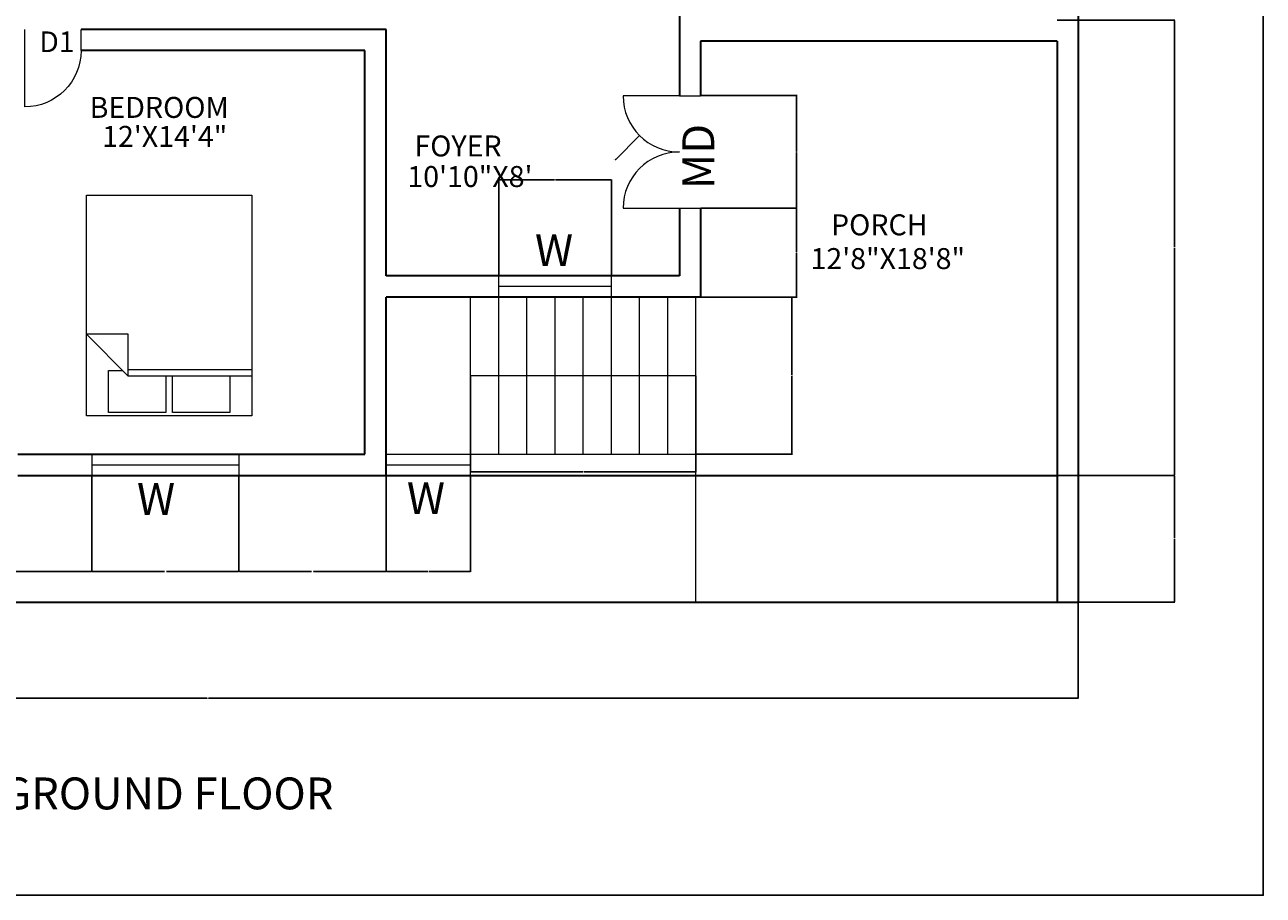
# Model space of a CAD drawing. Units: feet. Extents: x 1755 to 2628, y 1710 to 2329.
# Tile 2 of 4: x 2100 to 2628, y 1710 to 2081. Entities that reach past the tile are written whole.
import ezdxf

# ---------------------------------------------------------------- set-up
doc = ezdxf.new("R2010")
doc.units = ezdxf.units.FT
for name, color, linetype, lineweight in [('A-ANNO-DIMS', 2, 'Continuous', 18), ('A-ANNO-TEXT', 7, 'Continuous', 18), ('A-ANNO-TTLB', 7, 'Continuous', 25), ('A-AREA-IDEN', 7, 'Continuous', 18), ('A-DOOR', 3, 'Continuous', 18), ('A-FLOR-STRS', 7, 'Continuous', 18), ('A-FURN', 8, 'Continuous', 18), ('A-GLAZ', 4, 'Continuous', 18), ('A-WALL', 7, 'Continuous', 35)]:
    doc.layers.add(name, color=color, linetype=linetype, lineweight=lineweight)
doc.styles.get("Standard").update_dxf_attribs({"font": 'arial.ttf'})
doc.dimstyles.get("Standard").update_dxf_attribs({"dimtxt": 0.18, "dimasz": 0.18, "dimexe": 0.18, "dimexo": 0.0625, "dimgap": 0.09, "dimtad": 0, "dimtih": 1, "dimtoh": 1, "dimdec": 4, "dimzin": 0, "dimdsep": 46, "dimtxsty": 'Standard', "dimcen": 0.09, "dimadec": 0, "dimazin": 0, "dimtfac": 1, "dimtdec": 4, "dimtofl": 0, "dimtmove": 0, "dimatfit": 3, "dimfxl": 1, "dimtolj": 1, "dimtzin": 0, "dimarcsym": 0})

# ---------------------------------------------------------------- blocks, each defined once
blk = doc.blocks.new('Bed - Queen')
for p, q in [((0, -80.00003), (0, 0)), ((0, 0), (59.99999, 0)), ((59.99999, 0), (59.99999, -80.00003)), ((7.99999, -1.2), (28.79998, -1.2)), ((7.99999, -14.4), (7.99999, -1.2)), ((28.79998, -1.2), (28.79998, -14.4)), ((31.19999, -1.2), (51.99999, -1.2)), ((31.19999, -14.4), (31.19999, -1.2)), ((51.99999, -1.2), (51.99999, -16.4)), ((0, -14.4), (44.8, -14.4)), ((44.8, -16.8), (0, -16.8)), ((59.99999, -29.6), (44.8, -14.4)), ((44.8, -14.4), (44.8, -29.6)), ((51.99999, -16.4), (46.79936, -16.4)), ((44.8, -29.6), (59.99999, -29.6)), ((59.99999, -80.00003), (0, -80.00003))]:
    blk.add_line(p, q)
blk = doc.blocks.new('DOOR-SINGLE-SWING')
for p, q in [((0, 33), (0, 0)), ((24, 9), (24, 0))]:
    blk.add_line(p, q)
blk.add_arc((0, 9), 24, 0, 90)
blk = doc.blocks.new('*D22')
at = {"layer": 'A-ANNO-DIMS', "color": 0, "lineweight": -2, "transparency": 16777216}
for p, q in [((1806.89, 1834.75), (1806.89, 1793.69)), ((2548.89, 1834.75), (2548.89, 1793.69)), ((1807.07, 1793.87), (2177.6, 1793.87)), ((2548.71, 1793.87), (2178.18, 1793.87))]:
    blk.add_line(p, q, dxfattribs=at)
at = {"layer": 'A-ANNO-DIMS', "color": 0, "transparency": 16777216}
for points in [[(1807.07, 1793.9), (1807.07, 1793.84), (1806.89, 1793.87)], [(2548.71, 1793.9), (2548.71, 1793.84), (2548.89, 1793.87)]]:
    blk.add_solid(points, dxfattribs=at)
at = {"layer": 'Defpoints', "color": 0, "transparency": 16777216}
for p in [(1806.89, 1834.82), (2548.89, 1834.82), (2548.89, 1793.87)]:
    blk.add_point(p, dxfattribs=at)
at = {"layer": 'A-ANNO-DIMS', "color": 0, "transparency": 16777216, "insert": (2177.89, 1793.87), "char_height": 0.18, "attachment_point": 5}
blk.add_mtext('\\A1;742', dxfattribs=at)
blk = doc.blocks.new('*D34')
at = {"layer": 'A-ANNO-DIMS', "color": 0, "lineweight": -2, "transparency": 16777216}
for p, q in [((2539.95, 2082.82), (2590.02, 2082.82)), ((2589.84, 2082.64), (2589.84, 1986)), ((2589.84, 1889), (2589.84, 1985.63)), ((2539.95, 1888.82), (2590.02, 1888.82))]:
    blk.add_line(p, q, dxfattribs=at)
at = {"layer": 'A-ANNO-DIMS', "color": 0, "transparency": 16777216}
for points in [[(2589.81, 2082.64), (2589.87, 2082.64), (2589.84, 2082.82)], [(2589.81, 1889), (2589.87, 1889), (2589.84, 1888.82)]]:
    blk.add_solid(points, dxfattribs=at)
at = {"layer": 'Defpoints', "color": 0, "transparency": 16777216}
for p in [(2539.89, 2082.82), (2539.89, 1888.82), (2589.84, 1888.82)]:
    blk.add_point(p, dxfattribs=at)
at = {"layer": 'A-ANNO-DIMS', "color": 0, "transparency": 16777216, "insert": (2589.84, 1985.82), "char_height": 0.18, "attachment_point": 5}
blk.add_mtext('\\A1;194', dxfattribs=at)
blk = doc.blocks.new('*D35')
at = {"layer": 'A-ANNO-DIMS', "color": 0, "lineweight": -2, "transparency": 16777216}
for p, q in [((2539.95, 1888.82), (2590.02, 1888.82)), ((2589.84, 1888.64), (2589.84, 1862)), ((2589.84, 1835), (2589.84, 1861.63)), ((2539.95, 1834.82), (2590.02, 1834.82))]:
    blk.add_line(p, q, dxfattribs=at)
at = {"layer": 'A-ANNO-DIMS', "color": 0, "transparency": 16777216}
for points in [[(2589.81, 1888.64), (2589.87, 1888.64), (2589.84, 1888.82)], [(2589.81, 1835), (2589.87, 1835), (2589.84, 1834.82)]]:
    blk.add_solid(points, dxfattribs=at)
at = {"layer": 'Defpoints', "color": 0, "transparency": 16777216}
for p in [(2539.89, 1888.82), (2539.89, 1834.82), (2589.84, 1834.82)]:
    blk.add_point(p, dxfattribs=at)
at = {"layer": 'A-ANNO-DIMS', "color": 0, "transparency": 16777216, "insert": (2589.84, 1861.82), "char_height": 0.18, "attachment_point": 5}
blk.add_mtext('\\A1;54', dxfattribs=at)
blk = doc.blocks.new('*D40')
at = {"layer": 'A-ANNO-DIMS', "color": 0, "lineweight": -2, "transparency": 16777216}
for p, q in [((2035.77, 1888.75), (2035.77, 1847.69)), ((2128.5, 1888.75), (2128.5, 1847.69)), ((2035.95, 1847.87), (2081.75, 1847.87)), ((2128.32, 1847.87), (2082.53, 1847.87))]:
    blk.add_line(p, q, dxfattribs=at)
at = {"layer": 'A-ANNO-DIMS', "color": 0, "transparency": 16777216}
for points in [[(2035.95, 1847.9), (2035.95, 1847.84), (2035.77, 1847.87)], [(2128.32, 1847.9), (2128.32, 1847.84), (2128.5, 1847.87)]]:
    blk.add_solid(points, dxfattribs=at)
at = {"layer": 'Defpoints', "color": 0, "transparency": 16777216}
for p in [(2035.77, 1888.82), (2128.5, 1888.82), (2035.77, 1847.87)]:
    blk.add_point(p, dxfattribs=at)
at = {"layer": 'A-ANNO-DIMS', "color": 0, "transparency": 16777216, "insert": (2082.14, 1847.87), "char_height": 0.18, "attachment_point": 5}
blk.add_mtext('\\A1;92.73', dxfattribs=at)
blk = doc.blocks.new('*D41')
at = {"layer": 'A-ANNO-DIMS', "color": 0, "lineweight": -2, "transparency": 16777216}
for p, q in [((2128.5, 1888.75), (2128.5, 1847.69)), ((2191.17, 1888.75), (2191.17, 1847.69)), ((2128.68, 1847.87), (2159.44, 1847.87)), ((2190.99, 1847.87), (2160.23, 1847.87))]:
    blk.add_line(p, q, dxfattribs=at)
at = {"layer": 'A-ANNO-DIMS', "color": 0, "transparency": 16777216}
for points in [[(2128.68, 1847.9), (2128.68, 1847.84), (2128.5, 1847.87)], [(2190.99, 1847.9), (2190.99, 1847.84), (2191.17, 1847.87)]]:
    blk.add_solid(points, dxfattribs=at)
at = {"layer": 'Defpoints', "color": 0, "transparency": 16777216}
for p in [(2128.5, 1888.82), (2191.17, 1888.82), (2128.5, 1847.87)]:
    blk.add_point(p, dxfattribs=at)
at = {"layer": 'A-ANNO-DIMS', "color": 0, "transparency": 16777216, "insert": (2159.83, 1847.87), "char_height": 0.18, "attachment_point": 5}
blk.add_mtext('\\A1;62.66', dxfattribs=at)
blk = doc.blocks.new('*D42')
at = {"layer": 'A-ANNO-DIMS', "color": 0, "lineweight": -2, "transparency": 16777216}
for p, q in [((2191.17, 1888.75), (2191.17, 1847.69)), ((2253.89, 1888.75), (2253.89, 1847.69)), ((2191.35, 1847.87), (2222.13, 1847.87)), ((2253.71, 1847.87), (2222.92, 1847.87))]:
    blk.add_line(p, q, dxfattribs=at)
at = {"layer": 'A-ANNO-DIMS', "color": 0, "transparency": 16777216}
for points in [[(2191.35, 1847.9), (2191.35, 1847.84), (2191.17, 1847.87)], [(2253.71, 1847.9), (2253.71, 1847.84), (2253.89, 1847.87)]]:
    blk.add_solid(points, dxfattribs=at)
at = {"layer": 'Defpoints', "color": 0, "transparency": 16777216}
for p in [(2191.17, 1888.82), (2253.89, 1888.82), (2191.17, 1847.87)]:
    blk.add_point(p, dxfattribs=at)
at = {"layer": 'A-ANNO-DIMS', "color": 0, "transparency": 16777216, "insert": (2222.53, 1847.87), "char_height": 0.18, "attachment_point": 5}
blk.add_mtext('\\A1;62.73', dxfattribs=at)
blk = doc.blocks.new('*D43')
at = {"layer": 'A-ANNO-DIMS', "color": 0, "lineweight": -2, "transparency": 16777216}
for p, q in [((2253.89, 1888.75), (2253.89, 1847.69)), ((2289.89, 1888.75), (2289.89, 1847.69)), ((2254.07, 1847.87), (2271.67, 1847.87)), ((2289.71, 1847.87), (2272.11, 1847.87))]:
    blk.add_line(p, q, dxfattribs=at)
at = {"layer": 'A-ANNO-DIMS', "color": 0, "transparency": 16777216}
for points in [[(2254.07, 1847.9), (2254.07, 1847.84), (2253.89, 1847.87)], [(2289.71, 1847.9), (2289.71, 1847.84), (2289.89, 1847.87)]]:
    blk.add_solid(points, dxfattribs=at)
at = {"layer": 'Defpoints', "color": 0, "transparency": 16777216}
for p in [(2253.89, 1888.82), (2289.89, 1888.82), (2253.89, 1847.87)]:
    blk.add_point(p, dxfattribs=at)
at = {"layer": 'A-ANNO-DIMS', "color": 0, "transparency": 16777216, "insert": (2271.89, 1847.87), "char_height": 0.18, "attachment_point": 5}
blk.add_mtext('\\A1;36', dxfattribs=at)
blk = doc.blocks.new('*D44')
at = {"layer": 'A-ANNO-DIMS', "color": 0, "lineweight": -2, "transparency": 16777216}
for p, q in [((2289.89, 1931.25), (2289.89, 1890.19)), ((2385.89, 1931.25), (2385.89, 1890.19)), ((2290.07, 1890.37), (2337.67, 1890.37)), ((2385.71, 1890.37), (2338.11, 1890.37))]:
    blk.add_line(p, q, dxfattribs=at)
at = {"layer": 'A-ANNO-DIMS', "color": 0, "transparency": 16777216}
for points in [[(2290.07, 1890.4), (2290.07, 1890.34), (2289.89, 1890.37)], [(2385.71, 1890.4), (2385.71, 1890.34), (2385.89, 1890.37)]]:
    blk.add_solid(points, dxfattribs=at)
at = {"layer": 'Defpoints', "color": 0, "transparency": 16777216}
for p in [(2289.89, 1931.32), (2385.89, 1931.32), (2289.89, 1890.37)]:
    blk.add_point(p, dxfattribs=at)
at = {"layer": 'A-ANNO-DIMS', "color": 0, "transparency": 16777216, "insert": (2337.89, 1890.37), "char_height": 0.18, "attachment_point": 5}
blk.add_mtext('\\A1;96', dxfattribs=at)
blk = doc.blocks.new('*D45')
at = {"layer": 'A-ANNO-DIMS', "color": 0, "lineweight": -2, "transparency": 16777216}
for p, q in [((2385.95, 1964.82), (2427.02, 1964.82)), ((2426.84, 1964.64), (2426.84, 1931.5)), ((2426.84, 1898), (2426.84, 1931.13)), ((2385.95, 1897.82), (2427.02, 1897.82))]:
    blk.add_line(p, q, dxfattribs=at)
at = {"layer": 'A-ANNO-DIMS', "color": 0, "transparency": 16777216}
for points in [[(2426.81, 1964.64), (2426.87, 1964.64), (2426.84, 1964.82)], [(2426.81, 1898), (2426.87, 1898), (2426.84, 1897.82)]]:
    blk.add_solid(points, dxfattribs=at)
at = {"layer": 'Defpoints', "color": 0, "transparency": 16777216}
for p in [(2385.89, 1964.82), (2385.89, 1897.82), (2426.84, 1897.82)]:
    blk.add_point(p, dxfattribs=at)
at = {"layer": 'A-ANNO-DIMS', "color": 0, "transparency": 16777216, "insert": (2426.84, 1931.32), "char_height": 0.18, "attachment_point": 5}
blk.add_mtext('\\A1;67', dxfattribs=at)
blk = doc.blocks.new('*D46')
at = {"layer": 'A-ANNO-DIMS', "color": 0, "lineweight": -2, "transparency": 16777216}
for p, q in [((2387.95, 2050.61), (2429.02, 2050.61)), ((2428.84, 2050.43), (2428.84, 2026.79)), ((2428.84, 2002.79), (2428.84, 2026.43)), ((2387.95, 2002.61), (2429.02, 2002.61))]:
    blk.add_line(p, q, dxfattribs=at)
at = {"layer": 'A-ANNO-DIMS', "color": 0, "transparency": 16777216}
for points in [[(2428.81, 2050.43), (2428.87, 2050.43), (2428.84, 2050.61)], [(2428.81, 2002.79), (2428.87, 2002.79), (2428.84, 2002.61)]]:
    blk.add_solid(points, dxfattribs=at)
at = {"layer": 'Defpoints', "color": 0, "transparency": 16777216}
for p in [(2387.89, 2050.61), (2387.89, 2002.61), (2428.84, 2002.61)]:
    blk.add_point(p, dxfattribs=at)
at = {"layer": 'A-ANNO-DIMS', "color": 0, "transparency": 16777216, "insert": (2428.84, 2026.61), "char_height": 0.18, "attachment_point": 5}
blk.add_mtext('\\A1;48', dxfattribs=at)
blk = doc.blocks.new('*D47')
at = {"layer": 'A-ANNO-DIMS', "color": 0, "lineweight": -2, "transparency": 16777216}
for p, q in [((2387.95, 2002.61), (2429.02, 2002.61)), ((2428.84, 2002.43), (2428.84, 1983.89)), ((2428.84, 1965), (2428.84, 1983.53)), ((2387.95, 1964.82), (2429.02, 1964.82))]:
    blk.add_line(p, q, dxfattribs=at)
at = {"layer": 'A-ANNO-DIMS', "color": 0, "transparency": 16777216}
for points in [[(2428.81, 2002.43), (2428.87, 2002.43), (2428.84, 2002.61)], [(2428.81, 1965), (2428.87, 1965), (2428.84, 1964.82)]]:
    blk.add_solid(points, dxfattribs=at)
at = {"layer": 'Defpoints', "color": 0, "transparency": 16777216}
for p in [(2387.89, 2002.61), (2387.89, 1964.82), (2428.84, 1964.82)]:
    blk.add_point(p, dxfattribs=at)
at = {"layer": 'A-ANNO-DIMS', "color": 0, "transparency": 16777216, "insert": (2428.84, 1983.71), "char_height": 0.18, "attachment_point": 5}
blk.add_mtext('\\A1;37.79', dxfattribs=at)
blk = doc.blocks.new('*D48')
at = {"layer": 'A-ANNO-DIMS', "color": 0, "lineweight": -2, "transparency": 16777216}
for p, q in [((2301.89, 1973.88), (2301.89, 2014.95)), ((2302.07, 2014.77), (2325.67, 2014.77)), ((2349.71, 2014.77), (2326.11, 2014.77)), ((2349.89, 1973.88), (2349.89, 2014.95))]:
    blk.add_line(p, q, dxfattribs=at)
at = {"layer": 'A-ANNO-DIMS', "color": 0, "transparency": 16777216}
for points in [[(2302.07, 2014.8), (2302.07, 2014.74), (2301.89, 2014.77)], [(2349.71, 2014.8), (2349.71, 2014.74), (2349.89, 2014.77)]]:
    blk.add_solid(points, dxfattribs=at)
at = {"layer": 'Defpoints', "color": 0, "transparency": 16777216}
for p in [(2349.89, 2014.77), (2301.89, 1973.82), (2349.89, 1973.82)]:
    blk.add_point(p, dxfattribs=at)
at = {"layer": 'A-ANNO-DIMS', "color": 0, "transparency": 16777216, "insert": (2325.89, 2014.77), "char_height": 0.18, "attachment_point": 5}
blk.add_mtext('\\A1;48', dxfattribs=at)
blk = doc.blocks.new('*D54')
at = {"layer": 'A-ANNO-DIMS', "color": 0, "lineweight": -2, "transparency": 16777216}
for p, q in [((2378.8, 2050.61), (2378.98, 2050.61)), ((2378.89, 2050.52), (2378.89, 2050.7)), ((2351.74, 2023.45), (2361.79, 2033.51)), ((2351.56, 2023.45), (2351.74, 2023.45))]:
    blk.add_line(p, q, dxfattribs=at)
at = {"layer": 'A-ANNO-DIMS', "color": 0, "transparency": 16777216}
blk.add_solid([(2361.77, 2033.53), (2361.81, 2033.49), (2361.92, 2033.64)], dxfattribs=at)
at = {"layer": 'Defpoints', "color": 0, "transparency": 16777216}
for p in [(2378.89, 2050.61), (2361.92, 2033.64)]:
    blk.add_point(p, dxfattribs=at)
at = {"layer": 'A-ANNO-DIMS', "color": 0, "transparency": 16777216, "insert": (2351.06, 2023.45), "char_height": 0.18, "attachment_point": 5}
blk.add_mtext('\\A1;4X R24', dxfattribs=at)

msp = doc.modelspace()

# ---------------------------------------------------------------- linework, layer by layer
at = {"layer": 'A-ANNO-TTLB'}
msp.add_lwpolyline([(1754.8706, 2328.9307), (2627.7013, 2328.9307), (2627.7013, 1709.9251), (1754.8706, 1709.9251)], close=True, dxfattribs=at)
at = {"layer": 'A-DOOR'}
for p, q in [((2378.8905, 2050.608), (2354.8905, 2050.608)), ((2378.8905, 2050.608), (2387.8905, 2050.608)), ((2354.8905, 2002.608), (2387.8905, 2002.608))]:
    msp.add_line(p, q, dxfattribs=at)
for centre, start, end in [((2378.8905, 2050.608), 180, 270), ((2378.8905, 2002.608), 90, 180)]:
    msp.add_arc(centre, 24, start, end, dxfattribs=at)
at = {"layer": 'A-FLOR-STRS'}
for p, q in [((2301.8905, 1897.8157), (2301.8905, 1973.8157)), ((2349.8905, 1897.8157), (2349.8905, 1973.8157)), ((2289.8905, 1888.8157), (2289.8905, 1964.8157)), ((2313.8905, 1897.8157), (2313.8905, 1964.8157)), ((2325.8905, 1897.8157), (2325.8905, 1964.8157)), ((2337.8905, 1897.8157), (2337.8905, 1964.8157)), ((2361.8905, 1897.8157), (2361.8905, 1964.8157)), ((2373.8905, 1897.8157), (2373.8905, 1964.8157)), ((2385.8905, 1834.8157), (2385.8905, 1964.8157)), ((2289.8905, 1931.3157), (2385.8905, 1931.3157)), ((2253.8905, 1897.8157), (2385.8905, 1897.8157))]:
    msp.add_line(p, q, dxfattribs=at)
at = {"layer": 'A-GLAZ'}
for p, q in [((2349.8905, 1969.3157), (2301.8905, 1969.3157)), ((2128.5041, 1897.8157), (2128.5041, 1888.8157)), ((2191.1652, 1897.8157), (2191.1652, 1888.8157)), ((2128.5041, 1893.3157), (2191.1652, 1893.3157)), ((2253.8905, 1893.3157), (2289.8905, 1893.3157))]:
    msp.add_line(p, q, dxfattribs=at)
at = {"layer": 'A-WALL'}
for p, q in [((2548.8905, 2271.8157), (2548.8905, 1834.8157)), ((2378.8905, 2085.8157), (2378.8905, 2078.8157)), ((2244.8905, 2078.8157), (2123.8905, 2078.8157)), ((2253.8905, 2078.8157), (2238.3473, 2078.8157)), ((2253.8905, 1973.8157), (2253.8905, 2078.8157)), ((2378.8905, 2078.8157), (2378.8905, 2050.608)), ((2244.8905, 2069.8157), (2123.8905, 2069.8157)), ((2244.8905, 2069.8157), (2238.3473, 2069.8157)), ((2244.8905, 1897.8157), (2244.8905, 2069.8157)), ((2539.8905, 2073.8157), (2387.8905, 2073.8157)), ((2387.8905, 2073.8157), (2387.8905, 2050.608)), ((2539.8905, 2073.8157), (2539.8905, 1834.8157)), ((2378.8905, 2002.608), (2378.8905, 1973.8157)), ((2387.8905, 2002.608), (2387.8905, 1964.8157)), ((2378.8905, 1973.8157), (2253.8905, 1973.8157)), ((2253.8905, 1888.8157), (2253.8905, 1964.8157)), ((2387.8905, 1964.8157), (2253.8905, 1964.8157)), ((2096.8905, 1897.8157), (2244.8905, 1897.8157)), ((2096.8905, 1888.8157), (2244.8905, 1888.8157)), ((2244.8905, 1888.8157), (2539.8905, 1888.8157)), ((1806.8905, 1834.8157), (2548.8905, 1834.8157))]:
    msp.add_line(p, q, dxfattribs=at)

# ---------------------------------------------------------------- block references
at = {"layer": 'A-DOOR', "extrusion": (0, 0, -1), "zscale": -1, "rotation": 180}
msp.add_blockref('DOOR-SINGLE-SWING', (-2099.891, 2078.8153), dxfattribs=at)
at = {"layer": 'A-FURN', "xscale": 1.174519185879722, "yscale": 1.174519185879722, "zscale": 1.174519185879722, "rotation": 180}
msp.add_blockref('Bed - Queen', (2196.6327, 1914.1832), dxfattribs=at)

# ---------------------------------------------------------------- texts
at = {"layer": 'A-ANNO-TEXT'}
for s, height, p in [('D1', 8.79691, (2106.1248, 2069.1864)), ('W', 13.589, (2317.3163, 1977.965)), ('W', 13.589, (2147.6952, 1871.9893)), ('W', 13.589, (2262.7275, 1872.3197))]:
    msp.add_text(s, height=height, dxfattribs=at).set_placement(p)
msp.add_text('MD', height=13.58904, rotation=90, dxfattribs=at).set_placement((2393.7295, 2010.7718))
at = {"layer": 'A-ANNO-TTLB'}
msp.add_text('GROUND FLOOR', height=13.589045, dxfattribs=at).set_placement((2089.8587, 1746.5043))
at = {"layer": 'A-AREA-IDEN'}
for s, height, p in [('BEDROOM', 8.93153, (2127.539, 2041.1425)), ('12\'X14\'4"', 8.93153, (2132.8503, 2028.7794)), ('FOYER', 8.93153, (2265.9683, 2024.7068)), ('10\'10"X8\'', 8.93153, (2262.9323, 2011.6888)), ('PORCH', 8.93153, (2443.4946, 1991.1061)), ('12\'8"X18\'8"', 8.931529, (2434.7551, 1976.7219))]:
    msp.add_text(s, height=height, dxfattribs=at).set_placement(p)

# ---------------------------------------------------------------- dimensions: what is measured, and where the dimension line sits
at = {"layer": 'A-ANNO-DIMS'}
for base, p1, p2, angle, override, picture, middle in [((2589.8405, 1888.8157), (2539.8905, 2082.8157), (2539.8905, 1888.8157), 90, {"dimdec": 0, "dimlfac": 1, "dimrnd": 0, "dimzin": 0, "dimdsep": 46, "dimlunit": 2}, '*D34', (2589.8405, 1985.8157)), ((2428.8405, 2002.608), (2387.8905, 2050.608), (2387.8905, 2002.608), 270, {"dimdec": 0, "dimlfac": 1, "dimrnd": 0, "dimzin": 0, "dimdsep": 46, "dimlunit": 2}, '*D46', (2428.8405, 2026.608)), ((2428.8405, 1964.8157), (2387.8905, 2002.608), (2387.8905, 1964.8157), 270, {"dimdec": 2, "dimlfac": 1, "dimrnd": 0, "dimzin": 0, "dimdsep": 46, "dimlunit": 2}, '*D47', (2428.8405, 1983.7118)), ((2426.8405, 1897.8157), (2385.8905, 1964.8157), (2385.8905, 1897.8157), 270, {"dimdec": 0, "dimlfac": 1, "dimrnd": 0, "dimzin": 0, "dimdsep": 46, "dimlunit": 2}, '*D45', (2426.8405, 1931.3157)), ((2289.8905, 1890.3657), (2385.8905, 1931.3157), (2289.8905, 1931.3157), 180, {"dimdec": 0, "dimlfac": 1, "dimrnd": 0, "dimzin": 0, "dimdsep": 46, "dimlunit": 2}, '*D44', (2337.8905, 1890.3657)), ((2035.7745, 1847.8657), (2128.5041, 1888.8157), (2035.7745, 1888.8157), 180, {"dimdec": 2, "dimlfac": 1, "dimrnd": 0, "dimzin": 0, "dimdsep": 46, "dimlunit": 2}, '*D40', (2082.1393, 1847.8657)), ((2128.5041, 1847.8657), (2191.1652, 1888.8157), (2128.5041, 1888.8157), 180, {"dimdec": 2, "dimlfac": 1, "dimrnd": 0, "dimzin": 0, "dimdsep": 46, "dimlunit": 2}, '*D41', (2159.8347, 1847.8657)), ((2191.1652, 1847.8657), (2253.8905, 1888.8157), (2191.1652, 1888.8157), 180, {"dimdec": 2, "dimlfac": 1, "dimrnd": 0, "dimzin": 0, "dimdsep": 46, "dimlunit": 2}, '*D42', (2222.5279, 1847.8657)), ((2253.8905, 1847.8657), (2289.8905, 1888.8157), (2253.8905, 1888.8157), 180, {"dimdec": 0, "dimlfac": 1, "dimrnd": 0, "dimzin": 0, "dimdsep": 46, "dimlunit": 2}, '*D43', (2271.8905, 1847.8657)), ((2589.8405, 1834.8157), (2539.8905, 1888.8157), (2539.8905, 1834.8157), 90, {"dimdec": 0, "dimlfac": 1, "dimrnd": 0, "dimzin": 0, "dimdsep": 46, "dimlunit": 2}, '*D35', (2589.8405, 1861.8157))]:
    dim = msp.add_linear_dim(base=base, p1=p1, p2=p2, angle=angle, dimstyle='Standard', override=override, dxfattribs=at)
    dim.commit()
    dim.dimension.update_dxf_attribs({"geometry": picture, "text_midpoint": middle})
dim = msp.add_radius_dim(center=(2378.8905, 2050.608), mpoint=(2361.9202, 2033.6372), text='4X <>', dimstyle='Standard', override={"dimdec": 0, "dimlfac": 1, "dimrnd": 0, "dimzin": 0, "dimdsep": 46, "dimlunit": 2}, dxfattribs=at)
dim.commit()
dim.dimension.update_dxf_attribs({"geometry": '*D54', "text_midpoint": (2351.0563, 2023.4547), "dimtype": 164})
for base, p1, p2, picture, middle in [((2349.8905, 2014.7657), (2301.8905, 1973.8157), (2349.8905, 1973.8157), '*D48', (2325.8905, 2014.7657)), ((2548.8905, 1793.8657), (1806.8905, 1834.8157), (2548.8905, 1834.8157), '*D22', (2177.8905, 1793.8657))]:
    dim = msp.add_linear_dim(base=base, p1=p1, p2=p2, dimstyle='Standard', override={"dimdec": 0, "dimlfac": 1, "dimrnd": 0, "dimzin": 0, "dimdsep": 46, "dimlunit": 2}, dxfattribs=at)
    dim.commit()
    dim.dimension.update_dxf_attribs({"geometry": picture, "text_midpoint": middle})

doc.saveas('drawing.dxf')
